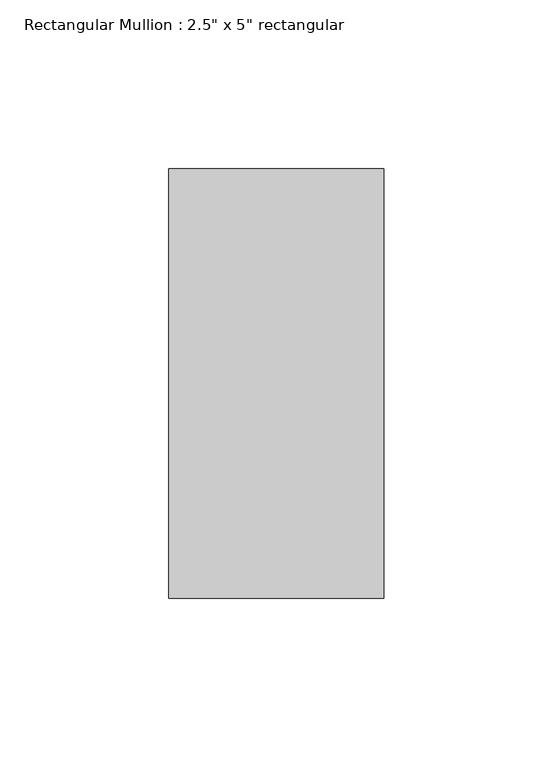
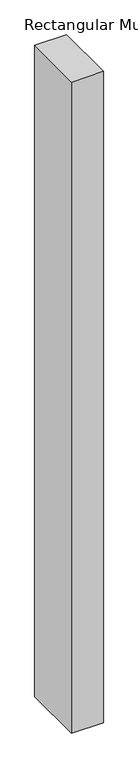
"""IFC4 building model written with IfcOpenShell, lengths in millimetres: member geometry."""

from ifc_helpers import new_model, si_unit, frame, origin, place, context, project, spatial, polyline, outline, extrude, source, transform, mapped, element, save


def member_bb3ab01a(model_context):
    return source(origin(), model_context, "Body", "SweptSolid", [
        extrude(outline(polyline([(0.0, 63.5), (0.0, -63.5), (-63.5, -63.5), (-63.5, 63.5), (0.0, 63.5)])), frame((0.0, 0.0, -1371.6000002), z_axis=(0.0, 0.0, 1.0), x_axis=(1.0, 0.0, 0.0)), (0.0, 0.0, 1.0), 1371.6000002),
    ])


if __name__ == "__main__":
    model = new_model("IFC4")
    model_context = context("Model", 3, world=origin())
    ifc_project = project(units=[si_unit("LENGTHUNIT", "METRE", prefix="MILLI")], contexts=[model_context])
    site = spatial("IfcSite", under=ifc_project)
    building = spatial("IfcBuilding", under=site)
    placement = place(None, origin())
    member_shape = member_bb3ab01a(model_context)
    element("IfcMember", 1, ObjectType="Rectangular Mullion : 2.5\" x 5\" rectangular", at=placement, inside=building, context=model_context, shape_type="MappedRepresentation", body=[
        mapped(member_shape, transform((0.0, 0.0, 0.0), x_axis=(1.0, 0.0, 0.0), y_axis=(0.0, 1.0, 0.0), z_axis=(0.0, 0.0, 1.0))),
    ])
    save(model, "model.ifc")

# Revit data of these elements
# Type "Rectangular Mullion : 2.5\" x 5\" rectangular"
#   built-in parameter 1007304 = 0.416667 (stored number, unit not read)
#   built-in parameter 1007301 = 0.104167 (stored number, unit not read)
#   built-in parameter 1007300 = 0.104167 (stored number, unit not read)
# Element 1 (IfcMember, "Rectangular Mullion : 2.5\" x 5\" rectangular")
#   Materials on its faces: "metal black"
# Materials
#   "metal black": class "Generic", colour RGB 120 120 120, transparency 0, Cost = 0
